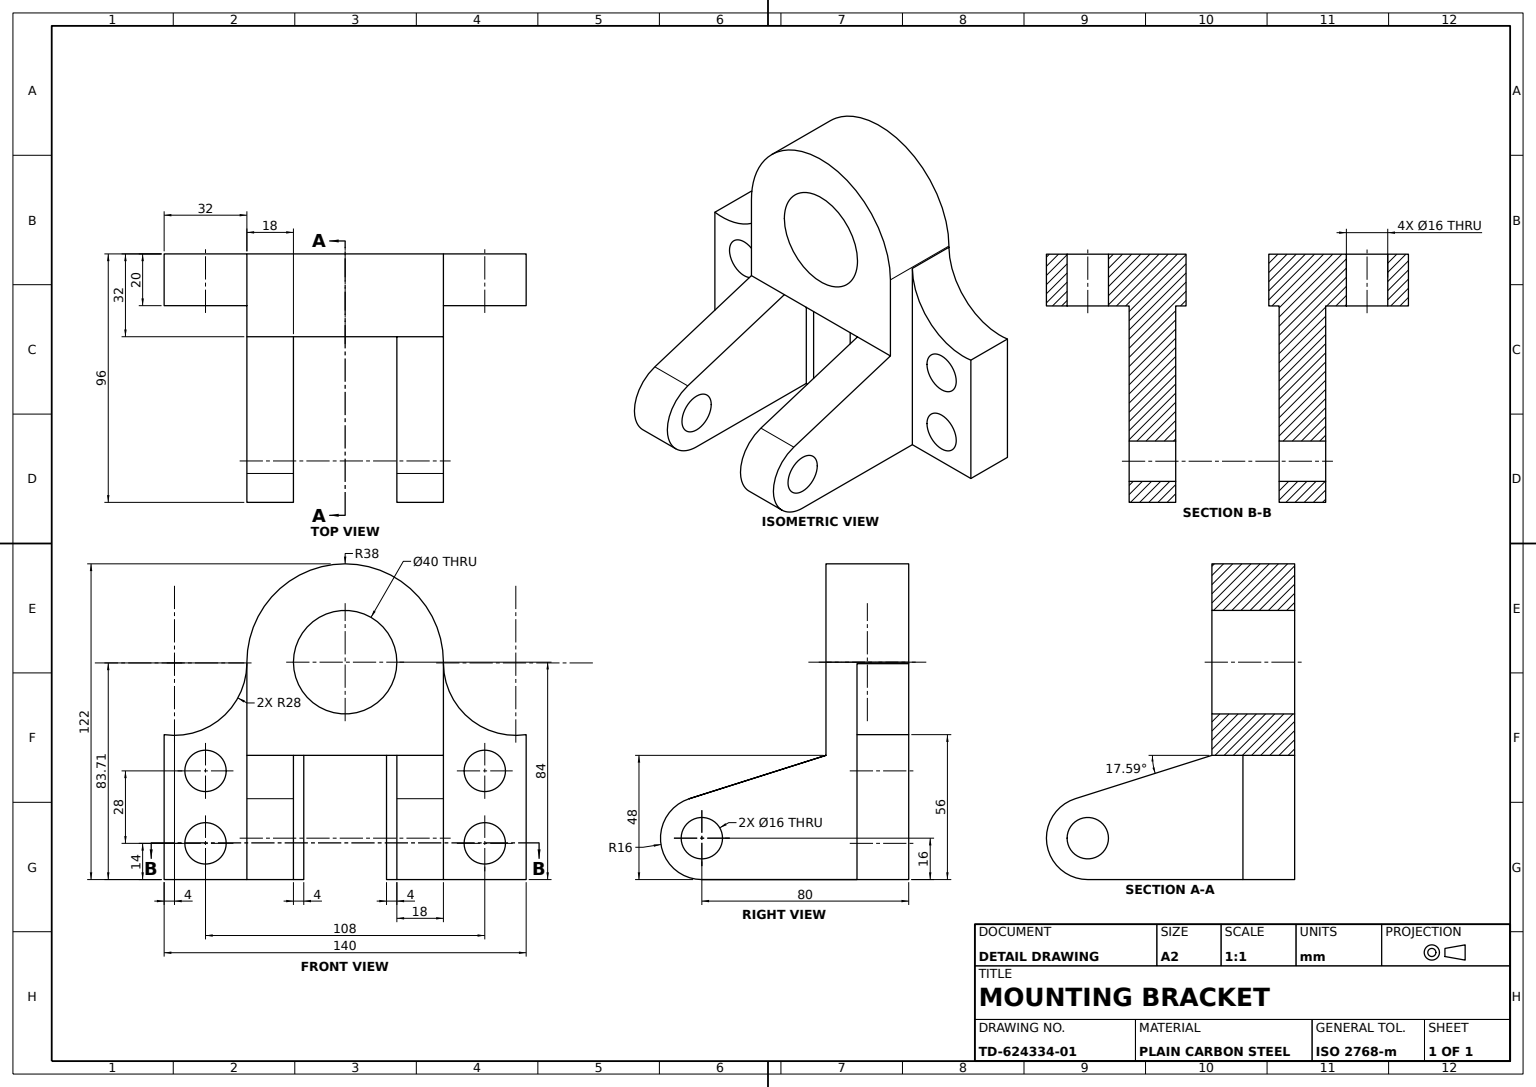
from build123d import *

# Parameters (mm, degrees)
HUB_PROFILE_SKETCH_R    = 20
HUB_BOSS_DEPTH          = 16
ARM_PROFILE_SKETCH_R    = 8
ARM_BOSS_DEPTH          = 18
FLANGE_PROFILE_SKETCH_R = 8
FLANGE_BOSS_DEPTH       = 20
WEB_PROFILE_SKETCH_W    = 4
WEB_PROFILE_SKETCH_H    = 48
WEB_BOSS_DEPTH          = 20


with BuildPart() as part:
    # Hub Profile Sketch → Hub Boss (new, symmetric)
    with BuildSketch(Plane(origin=(0, 0, 0), x_dir=(0, 0, -1), z_dir=(1, 0, 0))):
        with BuildLine():
            Line((-38, 0), (-38, -36))
            Line((-38, -36), (38, -36))
            Line((38, -36), (38, 0))
            ThreePointArc((38, 0), (0, 38), (-38, 0))
        make_face()
        Circle(HUB_PROFILE_SKETCH_R, mode=Mode.SUBTRACT)
    extrude(amount=HUB_BOSS_DEPTH, both=True)

    # Arm Profile Sketch → Arm Boss (add)
    with BuildSketch(Plane.XY.offset(38)):
        with BuildLine():
            ThreePointArc((68.834711668, -52.747932498), (79.811911333, -70.446111196), (64, -84))
            Line((64, -84), (-16, -84))
            Line((-16, -84), (-16, -36))
            Line((-16, -36), (16, -36))
            Line((16, -36), (68.834711668, -52.747932498))
        make_face()
        with Locations((64, -68)):
            Circle(ARM_PROFILE_SKETCH_R, mode=Mode.SUBTRACT)
    arm_boss = extrude(amount=-ARM_BOSS_DEPTH)

    # Arm Mirror: Arm Boss across plane
    add(arm_boss.mirror(Plane.XY))

    # Flange Profile Sketch → Flange Boss (add)
    with BuildSketch(Plane.ZY.offset(16)):
        with BuildLine():
            ThreePointArc((70, -28), (47.777657825, -21.547691645), (38, -0.574800039))
            Line((38, -0.574800039), (38, -84))
            Line((38, -84), (70, -84))
            Line((70, -84), (70, -28))
        make_face()
        with Locations((54, -70)):
            Circle(FLANGE_PROFILE_SKETCH_R, mode=Mode.SUBTRACT)
        with Locations((54, -42)):
            Circle(FLANGE_PROFILE_SKETCH_R, mode=Mode.SUBTRACT)
    flange_boss = extrude(amount=-FLANGE_BOSS_DEPTH)

    # Flange Mirror: Flange Boss across plane
    add(flange_boss.mirror(Plane.XY))

    # Web Profile Sketch → Web Boss (add)
    with BuildSketch(Plane.ZY.offset(16)):
        with Locations((-18, -60)):
            Rectangle(WEB_PROFILE_SKETCH_W, WEB_PROFILE_SKETCH_H)
    web_boss = extrude(amount=-WEB_BOSS_DEPTH)

    # Web Mirror: Web Boss across plane
    add(web_boss.mirror(Plane.XY))


solid = part.part
